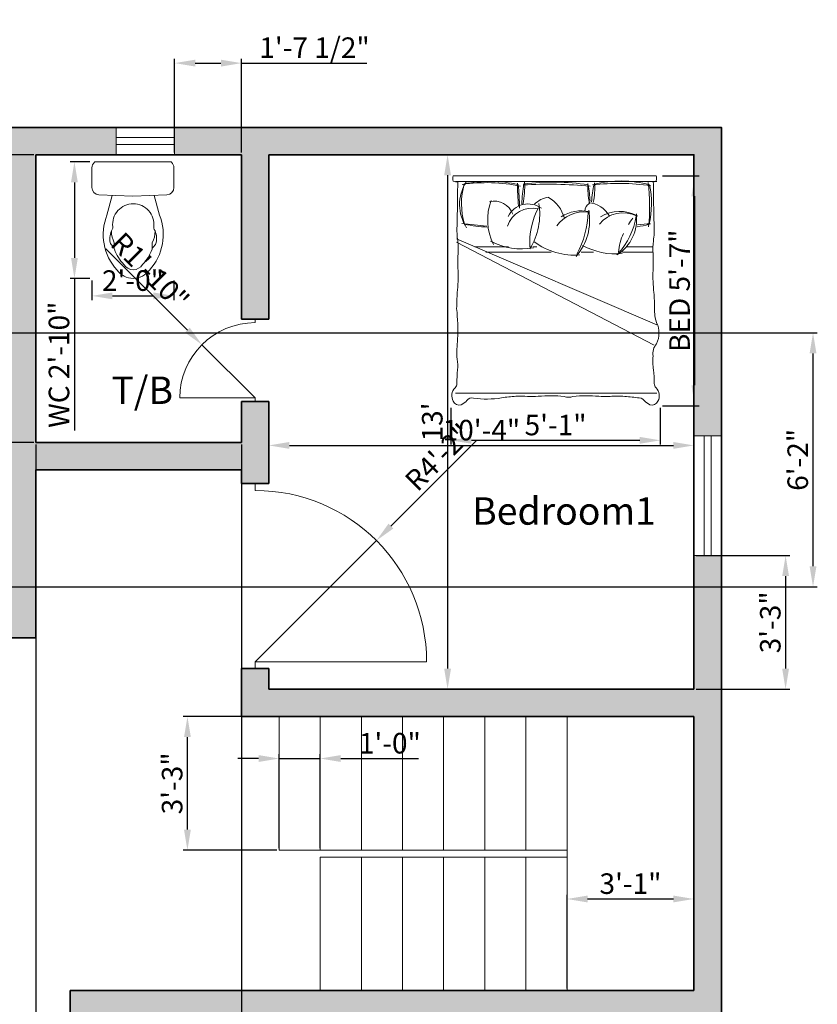
# Model space of a CAD drawing. Units: inches. Extents: x 2129 to 3258, y 1851 to 3021.
# Tile 7 of 10: x 2365 to 2598, y 2151 to 2439. Entities that reach past the tile are written whole.
import ezdxf

# ---------------------------------------------------------------- set-up
doc = ezdxf.new("R2010")
doc.units = ezdxf.units.IN
doc.linetypes.add('ACAD_ISO03W100', pattern=[30, 12, -18])
for name, color, linetype, lineweight in [('A-ANNO-DIMS', 2, 'Continuous', 18), ('A-AREA-IDEN', 7, 'Continuous', 20), ('A-DOOR', 4, 'Continuous', 18), ('A-FLOR-FIXT', 9, 'Continuous', 18), ('A-FLOR-STRS', 7, 'Continuous', 20), ('A-FURN', 8, 'Continuous', 18), ('A-GLAZ', 4, 'Continuous', 18), ('A-WALL', 7, 'Continuous', 35), ('A-WALL-OVHD', 8, 'ACAD_ISO03W100', 18)]:
    doc.layers.add(name, color=color, linetype=linetype, lineweight=lineweight)
doc.layers.add('A-WALL-PATT', color=32, linetype='Continuous', lineweight=13, true_color=0xcd6928)
doc.styles.get("Standard").update_dxf_attribs({"font": 'arial.ttf'})
doc.dimstyles.new('ISO-25', dxfattribs={"dimtxt": 6, "dimasz": 6, "dimexe": 1.25, "dimexo": 0.625, "dimtad": 1, "dimdec": 1, "dimlunit": 3, "dimtxsty": 'Standard', "dimcen": 2.5, "dimclrd": 5, "dimclre": 5, "dimadec": 0, "dimazin": 0, "dimtfac": 1, "dimtdec": 1, "dimtmove": 0, "dimatfit": 3, "dimfxl": 1, "dimarcsym": 0})

# ---------------------------------------------------------------- blocks, each defined once
blk = doc.blocks.new('A$C1308471B')
at = {"ltscale": 20}
for p, q in [((0, 0.4607), (0, 0.0186)), ((0.0354, 0.4793), (0.1495, 0.4793)), ((0.2013, 0.2397), (0.1923, 0.4384)), ((0.1957, 0.3639), (0.3109, 0.3953)), ((0.5021, 0.3528), (0.4724, 0.3528)), ((0.4982, 0.3575), (0.4822, 0.3709)), ((0.2013, 0.2397), (0.1923, 0.0409)), ((0.1959, 0.1193), (0.3109, 0.0879)), ((0.5021, 0.1304), (0.4724, 0.1304)), ((0.4982, 0.1257), (0.4822, 0.1123)), ((0.0354, 0), (0.1495, 0))]:
    blk.add_line(p, q, dxfattribs=at)
for centre, radius, start, end in [((0.006, 0.4607), 0.006, 136.52689, 180), ((0.0354, 0.4328), 0.0465, 90, 136.52689), ((0.1495, 0.4365), 0.0429, 2.57554, 90), ((0.4248, 0.1104), 0.3068, 47.41345, 111.79241), ((0.3654, 0.2416), 0.1206, 83.35226, 180), ((0.3823, 0.3868), 0.0255, 263.35226, 298.57415), ((0.4494, 0.2636), 0.1148, 79.39683, 118.57415), ((0.405, 0.2159), 0.153, 63.50202, 90.45216), ((0.4658, 0.3513), 0.0255, 50, 79.39683), ((0.5146, 0.377), 0.0255, 230, 251.38812), ((0.5021, 0.3273), 0.0255, 70.3751, 90), ((0.4248, 0.1104), 0.2558, 46.61198, 70.3751), ((0.5654, 0.2416), 0.065, 0, 57.29738), ((0.5654, 0.2416), 0.116, 0, 54.71147), ((0.3654, 0.2416), 0.1206, 180, 276.64774), ((0.5654, 0.2416), 0.065, 302.70262, 0), ((0.5654, 0.2416), 0.116, 305.28853, 0), ((0.4248, 0.3728), 0.2558, 289.6249, 313.38802), ((0.4248, 0.3728), 0.3068, 248.20759, 312.58655), ((0.3823, 0.0964), 0.0255, 61.42585, 96.64774), ((0.4494, 0.2196), 0.1148, 241.42585, 280.60317), ((0.405, 0.2673), 0.153, 269.54784, 296.49798), ((0.5146, 0.1062), 0.0255, 108.61188, 130), ((0.5021, 0.1559), 0.0255, 270, 289.6249), ((0.4658, 0.1319), 0.0255, 280.60317, 310), ((0.006, 0.0186), 0.006, 180, 223.47311), ((0.0354, 0.0465), 0.0465, 223.47311, 270), ((0.1495, 0.0429), 0.0429, 270, 357.42446)]:
    blk.add_arc(centre, radius, start, end, dxfattribs=at)
blk = doc.blocks.new('bed 1- king size')
at = {"color": 0}
for p, q in [((-0.9487, -0.0777), (0.9323, -0.0777)), ((-0.9394, -0.6151), (0.9323, -1.4177)), ((-0.9394, -0.6451), (0.9066, -1.6065)), ((-0.7682, -0.6873), (-0.4547, -0.6873)), ((-0.2254, -0.6873), (-0.1884, -0.6873)), ((0.6495, -0.6873), (0.8951, -0.6873)), ((-0.6659, -0.7381), (-0.0555, -0.7381)), ((0.2254, -0.7381), (0.3384, -0.7381)), ((0.6103, -0.7381), (0.8953, -0.7381)), ((-0.9487, -2.0547), (0.9323, -2.0547))]:
    blk.add_line(p, q, dxfattribs=at)
blk.add_lwpolyline([(0.898, -0.0829, 0.098699), (0.9236, -0.072, 0.222522), (0.9236, -0.0243), (-0.9705, -0.0243, 0.171621), (-0.9716, -0.0739, 0.102495), (-0.9268, -0.0829, 0.015571), (-0.9293, -0.2659, 0.00267), (-0.9341, -0.4944, 0.058958), (-0.9274, -0.6315, -0.038458), (-0.9248, -0.7552, 0.025508), (-0.9248, -0.9094, -0.039412), (-0.9326, -1.1154, 0.016498), (-0.9382, -1.2654, -0.035771), (-0.9288, -1.5502, 0.045388), (-0.9341, -1.7389, -0.080578), (-0.9295, -1.837, 0.026504), (-0.9362, -1.9656, -0.211134), (-0.9531, -2.0066, 0.329446), (-0.9701, -2.1314, 0.37589), (-0.8958, -2.1647, 0.123892), (-0.8425, -2.1233, -0.342539), (-0.78, -2.1029, 0.07104), (-0.5197, -2.1004, -0.036442), (-0.3847, -2.0853, -0.046791), (-0.2759, -2.0873, 0.023628), (-0.1759, -2.0852, -0.055897), (0.0662, -2.0877, 0.053528), (0.1067, -2.0945, 0.053528), (0.1472, -2.0877, -0.055897), (0.3893, -2.0852, 0.026973), (0.4769, -2.0873, -0.036947), (0.6147, -2.0853, -0.036442), (0.7497, -2.1004, -0.281256), (0.8137, -2.1233, -0.521995), (0.8137, -2.1233, 0.123892), (0.867, -2.1647, 0.37589), (0.9413, -2.1314, 0.329446), (0.9243, -2.0066, -0.211134), (0.9074, -1.9656, 0.026504), (0.9007, -1.837, -0.06219), (0.896, -1.7098, -0.218233), (0.9286, -1.5937, 0.123513), (0.9499, -1.4937, 0.129887), (0.9293, -1.3978, -0.095063), (0.9094, -1.2654, 0.016498), (0.9038, -1.1154, -0.039412), (0.896, -0.9094, 0.025508), (0.896, -0.7552, -0.038458), (0.8986, -0.6315, 0.058958), (0.9053, -0.4944, 0.00267), (0.9005, -0.2659, 0.015571)], format="xyb", close=True, dxfattribs=at)
for centre, radius, start, end in [((-0.5221, -0.2938), 0.3887, 147.50996, 213.83359), ((-0.6569, -1.6774), 1.5884, 78.54853, 98.3029), ((-0.6323, -1.3651), 1.2872, 78.01421, 100.51248), ((-1.2482, -0.1161), 0.9455, 349.58899, 2.04467), ((-0.04, -2.1818), 2.0978, 80.93396, 97.42659), ((0.5931, -1.1167), 1.0433, 75.01813, 103.73916), ((-1.0492, -0.3038), 1.9129, 354.09351, 6.47074), ((-0.2311, -0.2827), 0.6619, 163.92635, 197.14087), ((2.5431, -0.0869), 2.9129, 180.10628, 184.33117), ((-1.857, -0.3037), 1.5051, 359.15358, 7.55329), ((0.7071, -0.2897), 1.0355, 169.53013, 179.93405), ((-0.0818, -4.0689), 3.9654, 84.36579, 93.39687), ((1.0242, -0.1263), 0.7375, 177.82608, 191.47674), ((-0.6896, -0.2953), 0.9974, 1.8337, 10.6945), ((1.0572, -0.2894), 0.7358, 165.3434, 178.38757), ((0.5721, -2.1074), 2.0115, 81.37136, 96.91703), ((-0.3946, -0.1329), 0.7459, 349.16666, 3.12297), ((0.0089, -0.2863), 0.8722, 347.31751, 11.74345), ((-0.1358, -0.4371), 0.5128, 159.30257, 206.50263), ((-0.5846, -0.4421), 0.1803, 18.93869, 104.67251), ((-0.0546, -0.4435), 0.2189, 96.89924, 136.04208), ((-0.2438, -0.5051), 0.323, 15.40176, 59.7122), ((-0.2301, -0.5756), 0.2484, 78.04126, 160.83423), ((-0.2688, -0.4962), 0.2082, 54.16706, 153.84213), ((0.4039, -0.6426), 0.6595, 151.04555, 184.14969), ((-0.7873, -0.3825), 0.6248, 328.65419, 9.19769), ((0.2545, -0.6795), 0.3178, 83.56066, 144.28529), ((0.2294, -0.7137), 0.3612, 78.40806, 122.00775), ((-0.2123, -0.4404), 0.5157, 319.13389, 10.52989), ((-0.5982, -0.336), 0.8889, 331.60495, 358.1749), ((0.347, -0.3604), 0.0899, 120.11341, 175.89742), ((0.2786, -0.5137), 0.2374, 28.19956, 86.50605), ((0.5856, -0.7025), 0.345, 61.64039, 121.33448), ((0.6148, -0.6485), 0.2783, 61.88763, 141.87071), ((0.3458, -0.4294), 0.3969, 302.32623, 7.00001), ((0.0793, -0.3025), 0.6649, 317.32013, 351.4624), ((1.163, -0.8025), 0.5939, 139.95083, 146.95102), ((-1.8444, -10.4721), 10.046, 83.21322, 84.54762), ((-0.6059, 0.7469), 1.2515, 258.11692, 267.88493), ((0.6944, 0.0492), 0.5523, 275.44698, 287.41987), ((0.8799, -1.1936), 0.7214, 90.64318, 100.27066), ((-0.3293, -0.0779), 0.6301, 242.38587, 279.89508), ((0.1632, -0.137), 0.6293, 233.2201, 274.49725), ((1.163, -0.8025), 0.5939, 156.29818, 173.85386), ((0.5459, -0.118), 0.637, 240.94673, 275.46705)]:
    blk.add_arc(centre, radius, start, end, dxfattribs=at)
blk = doc.blocks.new('*D11')
at = {"layer": 'A-ANNO-DIMS', "color": 0, "lineweight": -2, "transparency": 16777216}
for p, q in [((2437.93, 2315.01), (2437.93, 2315.63)), ((2443.93, 2314.38), (2555.93, 2314.38)), ((2561.93, 2315.01), (2561.93, 2315.63))]:
    blk.add_line(p, q, dxfattribs=at)
at = {"layer": 'A-ANNO-DIMS', "color": 0, "transparency": 16777216}
for points in [[(2443.93, 2315.38), (2443.93, 2313.38), (2437.93, 2314.38)], [(2555.93, 2315.38), (2555.93, 2313.38), (2561.93, 2314.38)]]:
    blk.add_solid(points, dxfattribs=at)
at = {"layer": 'Defpoints', "color": 0, "transparency": 16777216}
for p in [(2437.93, 2314.38), (2561.93, 2314.38), (2561.93, 2314.38)]:
    blk.add_point(p, dxfattribs=at)
at = {"layer": 'A-ANNO-DIMS', "color": 0, "transparency": 16777216, "insert": (2499.93, 2318.07), "char_height": 6, "attachment_point": 5}
blk.add_mtext('10\'-4"', dxfattribs=at)
blk = doc.blocks.new('*D12')
at = {"layer": 'A-ANNO-DIMS', "color": 0, "lineweight": -2, "transparency": 16777216}
for p, q in [((2480.84, 2399.23), (2491.31, 2399.23)), ((2490.06, 2393.23), (2490.06, 2249.23)), ((2480.84, 2243.23), (2491.31, 2243.23))]:
    blk.add_line(p, q, dxfattribs=at)
at = {"layer": 'A-ANNO-DIMS', "color": 0, "transparency": 16777216}
for points in [[(2489.06, 2393.23), (2491.06, 2393.23), (2490.06, 2399.23)], [(2489.06, 2249.23), (2491.06, 2249.23), (2490.06, 2243.23)]]:
    blk.add_solid(points, dxfattribs=at)
at = {"layer": 'Defpoints', "color": 0, "transparency": 16777216}
for p in [(2480.22, 2399.23), (2480.22, 2243.23), (2490.06, 2243.23)]:
    blk.add_point(p, dxfattribs=at)
at = {"layer": 'A-ANNO-DIMS', "color": 0, "transparency": 16777216, "insert": (2486.37, 2321.23), "char_height": 6, "attachment_point": 5, "rotation": 90}
blk.add_mtext("13'", dxfattribs=at)
blk = doc.blocks.new('WIN-PLAN-35')
for p, q in [((0, 5), (35, 5)), ((0, 3), (35, 3))]:
    blk.add_line(p, q)
blk.add_lwpolyline([(0, 8), (35, 8), (35, 0), (0, 0)], close=True)
blk = doc.blocks.new('WIN-PLAN-17')
for p, q in [((0, 5), (17.03, 5)), ((0, 3), (17.03, 3))]:
    blk.add_line(p, q)
blk.add_lwpolyline([(0, 8), (17.03, 8), (17.03, 0), (0, 0)], close=True)
blk = doc.blocks.new('*D68')
at = {"layer": 'A-ANNO-DIMS', "color": 5, "lineweight": -2, "transparency": 16777216}
for p, q in [((2552.75, 2393.11), (2563.45, 2393.11)), ((2562.2, 2331.95), (2562.2, 2387.11)), ((2552.75, 2325.95), (2563.45, 2325.95))]:
    blk.add_line(p, q, dxfattribs=at)
at = {"layer": 'A-ANNO-DIMS', "color": 5, "transparency": 16777216}
for points in [[(2561.2, 2387.11), (2563.2, 2387.11), (2562.2, 2393.11)], [(2561.2, 2331.95), (2563.2, 2331.95), (2562.2, 2325.95)]]:
    blk.add_solid(points, dxfattribs=at)
at = {"layer": 'Defpoints', "color": 0, "transparency": 16777216}
for p in [(2552.13, 2393.11), (2562.2, 2393.11), (2552.13, 2325.95)]:
    blk.add_point(p, dxfattribs=at)
at = {"layer": 'A-ANNO-DIMS', "color": 0, "transparency": 16777216, "insert": (2558.52, 2359.53), "char_height": 6, "attachment_point": 5, "rotation": 90}
blk.add_mtext('BED 5\'-7"', dxfattribs=at)
blk = doc.blocks.new('*D69')
at = {"layer": 'A-ANNO-DIMS', "color": 5, "lineweight": -2, "transparency": 16777216}
for p, q in [((2491.01, 2325.32), (2491.01, 2314.62)), ((2552.13, 2325.32), (2552.13, 2314.62)), ((2497.01, 2315.87), (2546.13, 2315.87))]:
    blk.add_line(p, q, dxfattribs=at)
at = {"layer": 'A-ANNO-DIMS', "color": 5, "transparency": 16777216}
for points in [[(2497.01, 2316.87), (2497.01, 2314.87), (2491.01, 2315.87)], [(2546.13, 2316.87), (2546.13, 2314.87), (2552.13, 2315.87)]]:
    blk.add_solid(points, dxfattribs=at)
at = {"layer": 'Defpoints', "color": 0, "transparency": 16777216}
for p in [(2491.01, 2325.95), (2552.13, 2325.95), (2552.13, 2315.87)]:
    blk.add_point(p, dxfattribs=at)
at = {"layer": 'A-ANNO-DIMS', "color": 0, "transparency": 16777216, "insert": (2521.57, 2319.56), "char_height": 6, "attachment_point": 5}
blk.add_mtext('5\'-1"', dxfattribs=at)
blk = doc.blocks.new('*D74')
at = {"layer": 'A-ANNO-DIMS', "color": 5, "lineweight": -2, "transparency": 16777216}
for p, q in [((2385.67, 2397.15), (2379.94, 2397.15)), ((2381.19, 2391.15), (2381.19, 2369.14)), ((2385.67, 2363.14), (2379.94, 2363.14)), ((2381.19, 2363.14), (2381.19, 2318.74))]:
    blk.add_line(p, q, dxfattribs=at)
at = {"layer": 'A-ANNO-DIMS', "color": 5, "transparency": 16777216}
for points in [[(2380.19, 2391.15), (2382.19, 2391.15), (2381.19, 2397.15)], [(2380.19, 2369.14), (2382.19, 2369.14), (2381.19, 2363.14)]]:
    blk.add_solid(points, dxfattribs=at)
at = {"layer": 'Defpoints', "color": 0, "transparency": 16777216}
for p in [(2386.29, 2397.15), (2381.19, 2363.14), (2386.29, 2363.14)]:
    blk.add_point(p, dxfattribs=at)
at = {"layer": 'A-ANNO-DIMS', "color": 0, "transparency": 16777216, "insert": (2377.46, 2337.94), "char_height": 6, "attachment_point": 5, "rotation": 90}
blk.add_mtext('WC 2\'-10"', dxfattribs=at)
blk = doc.blocks.new('*D75')
at = {"layer": 'A-ANNO-DIMS', "color": 5, "lineweight": -2, "transparency": 16777216}
for p, q in [((2386.29, 2362.51), (2386.29, 2356.78)), ((2410.22, 2362.51), (2410.22, 2356.78)), ((2392.29, 2358.03), (2404.22, 2358.03))]:
    blk.add_line(p, q, dxfattribs=at)
at = {"layer": 'A-ANNO-DIMS', "color": 5, "transparency": 16777216}
for points in [[(2392.29, 2359.03), (2392.29, 2357.03), (2386.29, 2358.03)], [(2404.22, 2359.03), (2404.22, 2357.03), (2410.22, 2358.03)]]:
    blk.add_solid(points, dxfattribs=at)
at = {"layer": 'Defpoints', "color": 0, "transparency": 16777216}
for p in [(2386.29, 2363.14), (2410.22, 2363.14), (2410.22, 2358.03)]:
    blk.add_point(p, dxfattribs=at)
at = {"layer": 'A-ANNO-DIMS', "color": 0, "transparency": 16777216, "insert": (2398.26, 2361.72), "char_height": 6, "attachment_point": 5}
blk.add_mtext('2\'-0"', dxfattribs=at)
blk = doc.blocks.new('*D91')
at = {"layer": 'A-ANNO-DIMS', "color": 5, "lineweight": -2, "transparency": 16777216}
for p, q in [((2369.93, 2314.61), (2369.93, 1851.23)), ((2429.93, 2314.61), (2429.93, 1851.23)), ((2375.93, 1852.48), (2423.93, 1852.48))]:
    blk.add_line(p, q, dxfattribs=at)
at = {"layer": 'A-ANNO-DIMS', "color": 5, "transparency": 16777216}
for points in [[(2375.93, 1853.48), (2375.93, 1851.48), (2369.93, 1852.48)], [(2423.93, 1853.48), (2423.93, 1851.48), (2429.93, 1852.48)]]:
    blk.add_solid(points, dxfattribs=at)
at = {"layer": 'Defpoints', "color": 0, "transparency": 16777216}
for p in [(2369.93, 2315.23), (2429.93, 2315.23), (2429.93, 1852.48)]:
    blk.add_point(p, dxfattribs=at)
at = {"layer": 'A-ANNO-DIMS', "color": 0, "transparency": 16777216, "insert": (2399.93, 1856.17), "char_height": 6, "attachment_point": 5}
blk.add_mtext('5\'-0"', dxfattribs=at)
blk = doc.blocks.new('*D92')
at = {"layer": 'A-ANNO-DIMS', "color": 5, "lineweight": -2, "transparency": 16777216}
for p, q in [((2369.3, 2399.23), (2157.93, 2399.23)), ((2159.18, 2321.23), (2159.18, 2393.23)), ((2369.3, 2315.23), (2157.93, 2315.23))]:
    blk.add_line(p, q, dxfattribs=at)
at = {"layer": 'A-ANNO-DIMS', "color": 5, "transparency": 16777216}
for points in [[(2158.18, 2393.23), (2160.18, 2393.23), (2159.18, 2399.23)], [(2158.18, 2321.23), (2160.18, 2321.23), (2159.18, 2315.23)]]:
    blk.add_solid(points, dxfattribs=at)
at = {"layer": 'Defpoints', "color": 0, "transparency": 16777216}
for p in [(2159.18, 2399.23), (2369.93, 2399.23), (2369.93, 2315.23)]:
    blk.add_point(p, dxfattribs=at)
at = {"layer": 'A-ANNO-DIMS', "color": 0, "transparency": 16777216, "insert": (2155.49, 2357.23), "char_height": 6, "attachment_point": 5, "rotation": 90}
blk.add_mtext('7\'-0"', dxfattribs=at)
blk = doc.blocks.new('*D94')
at = {"layer": 'A-ANNO-DIMS', "color": 5, "lineweight": -2, "transparency": 16777216}
for p, q in [((2440.28, 2235.23), (2412.91, 2235.23)), ((2414.16, 2202.23), (2414.16, 2229.23)), ((2440.28, 2196.23), (2412.91, 2196.23))]:
    blk.add_line(p, q, dxfattribs=at)
at = {"layer": 'A-ANNO-DIMS', "color": 5, "transparency": 16777216}
for points in [[(2413.16, 2229.23), (2415.16, 2229.23), (2414.16, 2235.23)], [(2413.16, 2202.23), (2415.16, 2202.23), (2414.16, 2196.23)]]:
    blk.add_solid(points, dxfattribs=at)
at = {"layer": 'Defpoints', "color": 0, "transparency": 16777216}
for p in [(2414.16, 2235.23), (2440.91, 2235.23), (2440.91, 2196.23)]:
    blk.add_point(p, dxfattribs=at)
at = {"layer": 'A-ANNO-DIMS', "color": 0, "transparency": 16777216, "insert": (2410.47, 2215.73), "char_height": 6, "attachment_point": 5, "rotation": 90}
blk.add_mtext('3\'-3"', dxfattribs=at)
blk = doc.blocks.new('*D95')
at = {"layer": 'A-ANNO-DIMS', "color": 5, "lineweight": -2, "transparency": 16777216}
for p, q in [((2434.91, 2222.98), (2428.91, 2222.98)), ((2440.91, 2196.86), (2440.91, 2224.23)), ((2440.91, 2222.98), (2452.91, 2222.98)), ((2452.91, 2196.86), (2452.91, 2224.23)), ((2458.91, 2222.98), (2481.54, 2222.98))]:
    blk.add_line(p, q, dxfattribs=at)
at = {"layer": 'A-ANNO-DIMS', "color": 5, "transparency": 16777216}
for points in [[(2434.91, 2223.98), (2434.91, 2221.98), (2440.91, 2222.98)], [(2458.91, 2223.98), (2458.91, 2221.98), (2452.91, 2222.98)]]:
    blk.add_solid(points, dxfattribs=at)
at = {"layer": 'Defpoints', "color": 0, "transparency": 16777216}
for p in [(2452.91, 2222.98), (2440.91, 2196.23), (2452.91, 2196.23)]:
    blk.add_point(p, dxfattribs=at)
at = {"layer": 'A-ANNO-DIMS', "color": 0, "transparency": 16777216, "insert": (2473.22, 2226.67), "char_height": 6, "attachment_point": 5}
blk.add_mtext('1\'-0"', dxfattribs=at)
blk = doc.blocks.new('*D96')
at = {"layer": 'A-ANNO-DIMS', "color": 5, "lineweight": -2, "transparency": 16777216}
for p, q in [((2524.91, 2155.86), (2524.91, 2183.23)), ((2530.91, 2181.98), (2555.93, 2181.98)), ((2561.93, 2155.86), (2561.93, 2183.23))]:
    blk.add_line(p, q, dxfattribs=at)
at = {"layer": 'A-ANNO-DIMS', "color": 5, "transparency": 16777216}
for points in [[(2530.91, 2182.98), (2530.91, 2180.98), (2524.91, 2181.98)], [(2555.93, 2182.98), (2555.93, 2180.98), (2561.93, 2181.98)]]:
    blk.add_solid(points, dxfattribs=at)
at = {"layer": 'Defpoints', "color": 0, "transparency": 16777216}
for p in [(2561.93, 2181.98), (2524.91, 2155.23), (2561.93, 2155.23)]:
    blk.add_point(p, dxfattribs=at)
at = {"layer": 'A-ANNO-DIMS', "color": 0, "transparency": 16777216, "insert": (2543.42, 2185.68), "char_height": 6, "attachment_point": 5}
blk.add_mtext('3\'-1"', dxfattribs=at)
blk = doc.blocks.new('*D98')
at = {"layer": 'A-ANNO-DIMS', "color": 5, "lineweight": -2, "transparency": 16777216}
for p, q in [((2230.55, 2347.23), (2597.93, 2347.23)), ((2596.68, 2279.1), (2596.68, 2341.23)), ((2230.55, 2273.1), (2597.93, 2273.1))]:
    blk.add_line(p, q, dxfattribs=at)
at = {"layer": 'A-ANNO-DIMS', "color": 5, "transparency": 16777216}
for points in [[(2595.68, 2341.23), (2597.68, 2341.23), (2596.68, 2347.23)], [(2595.68, 2279.1), (2597.68, 2279.1), (2596.68, 2273.1)]]:
    blk.add_solid(points, dxfattribs=at)
at = {"layer": 'Defpoints', "color": 0, "transparency": 16777216}
for p in [(2229.93, 2347.23), (2596.68, 2347.23), (2229.93, 2273.1)]:
    blk.add_point(p, dxfattribs=at)
at = {"layer": 'A-ANNO-DIMS', "color": 0, "transparency": 16777216, "insert": (2592.99, 2310.17), "char_height": 6, "attachment_point": 5, "rotation": 90}
blk.add_mtext('6\'-2"', dxfattribs=at)
blk = doc.blocks.new('*D107')
at = {"layer": 'A-ANNO-DIMS', "color": 5, "lineweight": -2, "transparency": 16777216}
for p, q in [((2410.42, 2399.86), (2410.42, 2427.23)), ((2416.42, 2425.98), (2423.93, 2425.98)), ((2429.93, 2399.86), (2429.93, 2427.23)), ((2429.93, 2425.98), (2466.54, 2425.98))]:
    blk.add_line(p, q, dxfattribs=at)
at = {"layer": 'A-ANNO-DIMS', "color": 5, "transparency": 16777216}
for points in [[(2416.42, 2426.98), (2416.42, 2424.98), (2410.42, 2425.98)], [(2423.93, 2426.98), (2423.93, 2424.98), (2429.93, 2425.98)]]:
    blk.add_solid(points, dxfattribs=at)
at = {"layer": 'Defpoints', "color": 0, "transparency": 16777216}
for p in [(2429.93, 2425.98), (2410.42, 2399.23), (2429.93, 2399.23)]:
    blk.add_point(p, dxfattribs=at)
at = {"layer": 'A-ANNO-DIMS', "color": 0, "transparency": 16777216, "insert": (2451.24, 2429.71), "char_height": 6, "attachment_point": 5}
blk.add_mtext('1\'-7 1/2"', dxfattribs=at)
blk = doc.blocks.new('*D113')
at = {"layer": 'A-ANNO-DIMS', "color": 5, "lineweight": -2, "transparency": 16777216}
for p, q in [((2562.55, 2282.22), (2589.93, 2282.22)), ((2588.68, 2276.22), (2588.68, 2249.23)), ((2562.55, 2243.23), (2589.93, 2243.23))]:
    blk.add_line(p, q, dxfattribs=at)
at = {"layer": 'A-ANNO-DIMS', "color": 5, "transparency": 16777216}
for points in [[(2587.68, 2276.22), (2589.68, 2276.22), (2588.68, 2282.22)], [(2587.68, 2249.23), (2589.68, 2249.23), (2588.68, 2243.23)]]:
    blk.add_solid(points, dxfattribs=at)
at = {"layer": 'Defpoints', "color": 0, "transparency": 16777216}
for p in [(2561.93, 2282.22), (2561.93, 2243.23), (2588.68, 2243.23)]:
    blk.add_point(p, dxfattribs=at)
at = {"layer": 'A-ANNO-DIMS', "color": 0, "transparency": 16777216, "insert": (2584.99, 2262.73), "char_height": 6, "attachment_point": 5, "rotation": 90}
blk.add_mtext('3\'-3"', dxfattribs=at)
blk = doc.blocks.new('*D135')
at = {"layer": 'A-ANNO-DIMS', "color": 5, "lineweight": -2, "transparency": 16777216}
for p, q in [((2498.61, 2315.91), (2473.53, 2290.83)), ((2433.93, 2251.23), (2469.28, 2286.59))]:
    blk.add_line(p, q, dxfattribs=at)
at = {"layer": 'A-ANNO-DIMS', "color": 5, "transparency": 16777216}
blk.add_solid([(2472.82, 2291.54), (2474.23, 2290.13), (2469.28, 2286.59)], dxfattribs=at)
at = {"layer": 'Defpoints', "color": 0, "transparency": 16777216}
for p in [(2469.28, 2286.59), (2433.93, 2251.23)]:
    blk.add_point(p, dxfattribs=at)
at = {"layer": 'A-ANNO-DIMS', "color": 0, "transparency": 16777216, "insert": (2487.92, 2310.38), "char_height": 6, "attachment_point": 5, "rotation": 45.0003}
blk.add_mtext('R4\'-2"', dxfattribs=at)
blk = doc.blocks.new('*D139')
at = {"layer": 'A-ANNO-DIMS', "color": 5, "lineweight": -2, "transparency": 16777216}
for p, q in [((2390.38, 2371.81), (2414.13, 2348.04)), ((2433.93, 2328.23), (2418.38, 2343.79))]:
    blk.add_line(p, q, dxfattribs=at)
at = {"layer": 'A-ANNO-DIMS', "color": 5, "transparency": 16777216}
blk.add_solid([(2414.84, 2348.75), (2413.43, 2347.33), (2418.38, 2343.79)], dxfattribs=at)
at = {"layer": 'Defpoints', "color": 0, "transparency": 16777216}
for p in [(2418.38, 2343.79), (2433.93, 2328.23)]:
    blk.add_point(p, dxfattribs=at)
at = {"layer": 'A-ANNO-DIMS', "color": 0, "transparency": 16777216, "insert": (2402.74, 2364.65), "char_height": 6, "attachment_point": 5, "rotation": 314.9864}
blk.add_mtext('R1\'-10"', dxfattribs=at)

msp = doc.modelspace()

# ---------------------------------------------------------------- hatches: boundary and pattern name
at = {"layer": 'A-WALL-PATT'}
h = msp.add_hatch(color=256, dxfattribs=at)
h.dxf.hatch_style = 1
h.paths.add_polyline_path([(2393.39, 2407.23), (2185.93, 2407.23), (2185.93, 2394.06), (2193.93, 2394.06), (2193.93, 2399.23), (2361.93, 2399.23), (2361.93, 2355.23), (2361.93, 2347.23), (2361.93, 2258.25), (2369.93, 2258.25), (2369.93, 2307.23), (2429.93, 2307.23), (2429.93, 2303.23), (2437.93, 2303.23), (2437.93, 2327.23), (2429.93, 2327.23), (2429.93, 2315.23), (2369.93, 2315.23), (2369.93, 2399.23), (2393.39, 2399.23)])
h.paths.add_polyline_path([(2569.93, 2407.23), (2410.42, 2407.23), (2410.42, 2399.23), (2429.93, 2399.23), (2429.93, 2351.23), (2437.93, 2351.23), (2437.93, 2399.23), (2561.93, 2399.23), (2561.93, 2317.22), (2569.93, 2317.22)])
h.paths.add_polyline_path([(2569.93, 2282.22), (2561.93, 2282.22), (2561.93, 2243.23), (2437.93, 2243.23), (2437.93, 2249.23), (2429.93, 2249.23), (2429.93, 2235.23), (2561.93, 2235.23), (2561.93, 2155.23), (2379.93, 2155.23), (2379.93, 2147.23), (2385.93, 2147.23), (2385.93, 2141.23), (2393.93, 2141.23), (2393.93, 2147.23), (2469.93, 2147.23), (2469.93, 2111.23), (2477.93, 2111.23), (2477.93, 2147.23), (2561.93, 2147.23), (2561.93, 2129.53), (2569.93, 2129.53)])
h.paths.add_polyline_path([(2569.93, 2112.5), (2561.93, 2112.5), (2561.93, 2063.23), (2477.93, 2063.23), (2477.93, 2069.23), (2469.93, 2069.23), (2469.93, 2063.23), (2445.93, 2063.23), (2445.93, 2055.23), (2561.93, 2055.23), (2561.93, 1951.04), (2569.93, 1951.04)])
h.paths.add_polyline_path([(2569.93, 1916.04), (2561.93, 1916.04), (2561.93, 1887.23), (2393.93, 1887.23), (2393.93, 2055.23), (2399.93, 2055.23), (2399.93, 2063.23), (2393.93, 2063.23), (2393.93, 2087.23), (2385.93, 2087.23), (2385.93, 1887.23), (2385.93, 1879.23), (2569.93, 1879.23)])
h.paths.add_polyline_path([(2193.93, 2147.23), (2289.93, 2147.23), (2289.93, 2155.23), (2193.93, 2155.23), (2193.93, 2170.77), (2185.93, 2170.77), (2185.93, 2056.85), (2193.93, 2056.85)])
h.paths.add_polyline_path([(2193.93, 2021.85), (2185.93, 2021.85), (2185.93, 1959.23), (2222.56, 1959.23), (2222.56, 1967.23), (2193.93, 1967.23)])
h.paths.add_polyline_path([(2307.93, 1967.23), (2257.56, 1967.23), (2257.56, 1959.23), (2307.93, 1959.23)])
h.paths.add_polyline_path([(2255.61, 2368.18), (2321.09, 2368.18), (2321.09, 2384.66), (2255.61, 2384.66)], flags=25)
h.paths.add_polyline_path([(2282.89, 2032.34), (2325.27, 2032.34), (2325.27, 2051.27), (2282.89, 2051.27)], flags=9)
h.paths.add_polyline_path([(2404.09, 1945.18), (2463.36, 1945.18), (2463.36, 1961.66), (2404.09, 1961.66)], flags=25)
h.paths.add_polyline_path([(2494.41, 2286.84), (2553.68, 2286.84), (2553.68, 2303.32), (2494.41, 2303.32)], flags=9)
h.paths.add_polyline_path([(2389.71, 2321.98), (2411.09, 2321.98), (2411.09, 2338.47), (2389.71, 2338.47)], flags=25)
h.paths.add_polyline_path([(2219.41, 2162.82), (2258.18, 2162.82), (2258.18, 2179.3), (2219.41, 2179.3)], flags=9)
h.paths.add_polyline_path([(2249.68, 2306.23), (2298.12, 2306.23), (2298.12, 2323.98), (2249.68, 2323.98)], flags=25)
h = msp.add_hatch(color=256, dxfattribs=at)
h.dxf.hatch_style = 1
h.paths.add_polyline_path([(2193.93, 2288.35), (2185.93, 2288.35), (2185.93, 2205.77), (2193.93, 2205.77)])
h.paths.add_polyline_path([(2193.93, 2347.23), (2310.77, 2347.23), (2310.77, 2355.23), (2193.93, 2355.23), (2193.93, 2359.06), (2185.93, 2359.06), (2185.93, 2323.35), (2193.93, 2323.35)])
h.paths.add_polyline_path([(2314.44, 2244.01), (2314.44, 2257.94), (2302.07, 2257.94), (2302.07, 2244.01)], flags=9)
h.paths.add_polyline_path([(2255.61, 2368.18), (2321.09, 2368.18), (2321.09, 2384.66), (2255.61, 2384.66)], flags=9)
h.paths.add_polyline_path([(2282.89, 2032.34), (2325.27, 2032.34), (2325.27, 2051.27), (2282.89, 2051.27)], flags=9)
h.paths.add_polyline_path([(2404.09, 1945.18), (2463.36, 1945.18), (2463.36, 1961.66), (2404.09, 1961.66)], flags=9)
h.paths.add_polyline_path([(2494.41, 2286.84), (2553.68, 2286.84), (2553.68, 2303.32), (2494.41, 2303.32)], flags=9)
h.paths.add_polyline_path([(2389.71, 2321.98), (2411.09, 2321.98), (2411.09, 2338.47), (2389.71, 2338.47)], flags=9)
h.paths.add_polyline_path([(2219.41, 2162.82), (2258.18, 2162.82), (2258.18, 2179.3), (2219.41, 2179.3)], flags=9)
h.paths.add_polyline_path([(2249.68, 2306.23), (2298.12, 2306.23), (2298.12, 2323.98), (2249.68, 2323.98)], flags=9)

# ---------------------------------------------------------------- linework, layer by layer
at = {"layer": 'A-DOOR'}
for p, q in [((2433.93, 2351.23), (2433.93, 2350.23)), ((2433.93, 2328.23), (2411.93, 2328.23)), ((2433.93, 2327.23), (2433.93, 2328.23)), ((2433.93, 2303.23), (2433.93, 2301.23)), ((2433.93, 2249.23), (2433.93, 2251.23)), ((2433.93, 2251.23), (2483.93, 2251.23))]:
    msp.add_line(p, q, dxfattribs=at)
for centre, radius, start, end in [((2433.93, 2328.23), 22, 90, 180), ((2433.93, 2251.23), 50, 0, 90)]:
    msp.add_arc(centre, radius, start, end, dxfattribs=at)
at = {"layer": 'A-FLOR-STRS'}
for p, q in [((2440.91, 2235.23), (2440.91, 2196.23)), ((2452.91, 2235.23), (2452.91, 2196.23)), ((2464.91, 2235.23), (2464.91, 2196.23)), ((2476.91, 2235.23), (2476.91, 2196.23)), ((2488.91, 2196.23), (2488.91, 2235.23)), ((2500.91, 2235.23), (2500.91, 2196.23)), ((2512.91, 2235.23), (2512.91, 2196.23)), ((2524.91, 2235.23), (2524.91, 2194.23)), ((2524.91, 2196.23), (2440.91, 2196.23)), ((2524.91, 2194.23), (2452.91, 2194.23)), ((2452.91, 2194.23), (2452.91, 2155.23)), ((2464.91, 2194.23), (2464.91, 2155.23)), ((2476.91, 2194.23), (2476.91, 2155.23)), ((2488.91, 2194.23), (2488.91, 2155.23)), ((2500.91, 2194.23), (2500.91, 2155.23)), ((2512.91, 2194.23), (2512.91, 2155.23)), ((2524.91, 2194.23), (2524.91, 2155.23))]:
    msp.add_line(p, q, dxfattribs=at)
at = {"layer": 'A-WALL'}
for p, q in [((2369.93, 2399.23), (2369.93, 2315.23)), ((2429.93, 2399.23), (2429.93, 2351.23)), ((2437.93, 2399.23), (2437.93, 2351.23)), ((2437.93, 2399.23), (2561.93, 2399.23)), ((2429.93, 2351.23), (2437.93, 2351.23)), ((2429.93, 2327.23), (2437.93, 2327.23)), ((2429.93, 2327.23), (2429.93, 2315.23)), ((2437.93, 2327.23), (2437.93, 2303.23)), ((2369.93, 2315.23), (2429.93, 2315.23)), ((2369.93, 2307.23), (2429.93, 2307.23)), ((2369.93, 2307.23), (2369.93, 2258.25)), ((2429.93, 2307.23), (2429.93, 2303.23)), ((2429.93, 2303.23), (2437.93, 2303.23)), ((2361.93, 2258.25), (2369.93, 2258.25)), ((2437.93, 2249.23), (2429.93, 2249.23)), ((2429.93, 2249.23), (2429.93, 2235.23)), ((2437.93, 2249.23), (2437.93, 2243.23)), ((2437.93, 2243.23), (2561.93, 2243.23)), ((2429.93, 2235.23), (2561.93, 2235.23)), ((2561.93, 2235.23), (2561.93, 2155.23)), ((2379.93, 2147.23), (2379.93, 2155.23)), ((2379.93, 2155.23), (2561.93, 2155.23))]:
    msp.add_line(p, q, dxfattribs=at)
msp.add_lwpolyline([(2185.93, 2407.23), (2569.93, 2407.23), (2569.93, 1879.23), (2185.93, 1879.23)], close=True, dxfattribs=at)
for points in [[(2369.93, 2399.23), (2429.93, 2399.23)], [(2437.93, 2399.23), (2561.93, 2399.23), (2561.93, 2243.23)], [(2561.93, 2235.23), (2561.93, 2155.23)]]:
    msp.add_lwpolyline(points, dxfattribs=at)
at = {"layer": 'A-WALL-OVHD'}
msp.add_line((2289.93, 2155.23), (2379.93, 2155.23), dxfattribs=at)

# ---------------------------------------------------------------- block references
at = {"layer": 'A-FLOR-FIXT', "xscale": 49.91928435982494, "yscale": 49.91928435982494, "zscale": 49.91928435982494, "rotation": 269.9999999999996}
msp.add_blockref('A$C1308471B', (2386.29, 2397.15), dxfattribs=at)
at = {"layer": 'A-FURN', "xscale": 31.24411875038765, "yscale": 31.24411875038765, "zscale": 31.24411875038765}
msp.add_blockref('bed 1- king size', (2522.02, 2393.87), dxfattribs=at)
at = {"layer": 'A-GLAZ'}
msp.add_blockref('WIN-PLAN-17', (2393.39, 2399.24), dxfattribs=at)
at = {"layer": 'A-GLAZ', "rotation": 89.99999999999972}
msp.add_blockref('WIN-PLAN-35', (2569.93, 2282.22), dxfattribs=at)

# ---------------------------------------------------------------- texts
at = {"layer": 'A-AREA-IDEN', "char_height": 8, "attachment_point": 1}
for s, width, insert in [('T/B', 7.067, (2391.97, 2334.49)), ('{\\fArial|b1|i0|c0|p34;Bedroom1}', 58.4293, (2497.23, 2299.24))]:
    msp.add_mtext_dynamic_manual_height_columns(s, width=width, gutter_width=12.5, heights=[0], dxfattribs=dict(at, insert=insert))

# ---------------------------------------------------------------- dimensions: what is measured, and where the dimension line sits
at = {"layer": 'A-ANNO-DIMS'}
for base, p1, p2, override, picture, middle in [((2429.93, 2425.98), (2410.42, 2399.23), (2429.93, 2399.23), {"dimdec": 1, "dimlfac": 1, "dimrnd": 0, "dimzin": 1, "dimdsep": 46, "dimlunit": 4, "dimfrac": 2}, '*D107', (2451.24, 2429.71)), ((2410.22, 2358.03), (2386.29, 2363.14), (2410.22, 2363.14), {"dimdec": 1, "dimlfac": 1, "dimrnd": 0, "dimzin": 1, "dimdsep": 46, "dimlunit": 4, "dimfrac": 2}, '*D75', (2398.26, 2361.72)), ((2552.13, 2315.87), (2491.01, 2325.95), (2552.13, 2325.95), {"dimdec": 1, "dimlfac": 1, "dimrnd": 0, "dimzin": 1, "dimdsep": 46, "dimlunit": 4, "dimfrac": 2}, '*D69', (2521.57, 2319.56)), ((2561.93, 2314.38), (2437.93, 2314.38), (2561.93, 2314.38), {"dimclrd": 0, "dimclre": 0, "dimclrt": 0}, '*D11', (2499.93, 2318.07)), ((2429.93, 1852.48), (2369.93, 2315.23), (2429.93, 2315.23), {"dimdec": 1, "dimlfac": 1, "dimrnd": 0, "dimzin": 1, "dimdsep": 46, "dimlunit": 4, "dimfrac": 2}, '*D91', (2399.93, 1856.17)), ((2452.91, 2222.98), (2440.91, 2196.23), (2452.91, 2196.23), {"dimdec": 1, "dimlfac": 1, "dimrnd": 0, "dimzin": 1, "dimdsep": 46, "dimlunit": 4, "dimfrac": 2}, '*D95', (2473.22, 2226.67)), ((2561.93, 2181.98), (2524.91, 2155.23), (2561.93, 2155.23), {"dimdec": 1, "dimlfac": 1, "dimrnd": 0, "dimzin": 1, "dimdsep": 46, "dimlunit": 4, "dimfrac": 2}, '*D96', (2543.42, 2185.68))]:
    dim = msp.add_linear_dim(base=base, p1=p1, p2=p2, dimstyle='ISO-25', override=override, dxfattribs=at)
    dim.commit()
    dim.dimension.update_dxf_attribs({"geometry": picture, "text_midpoint": middle})
for base, p1, p2, angle, override, picture, middle in [((2159.18, 2399.23), (2369.93, 2315.23), (2369.93, 2399.23), 90, {"dimdec": 1, "dimlfac": 1, "dimrnd": 0, "dimzin": 1, "dimdsep": 46, "dimlunit": 4, "dimfrac": 2}, '*D92', (2155.49, 2357.23)), ((2490.06, 2243.23), (2480.22, 2399.23), (2480.22, 2243.23), 90, {"dimclrd": 0, "dimclre": 0, "dimclrt": 0}, '*D12', (2486.37, 2321.23)), ((2596.68, 2347.23), (2229.93, 2273.1), (2229.93, 2347.23), 90, {"dimdec": 1, "dimlfac": 1, "dimrnd": 0, "dimzin": 1, "dimdsep": 46, "dimlunit": 4, "dimfrac": 2}, '*D98', (2592.99, 2310.17)), ((2588.68, 2243.23), (2561.93, 2282.22), (2561.93, 2243.23), 270, {"dimdec": 1, "dimlfac": 1, "dimrnd": 0, "dimzin": 1, "dimdsep": 46, "dimlunit": 4, "dimfrac": 2}, '*D113', (2584.99, 2262.73)), ((2414.16, 2235.23), (2440.91, 2196.23), (2440.91, 2235.23), 90, {"dimdec": 1, "dimlfac": 1, "dimrnd": 0, "dimzin": 1, "dimdsep": 46, "dimlunit": 4, "dimfrac": 2}, '*D94', (2410.47, 2215.73))]:
    dim = msp.add_linear_dim(base=base, p1=p1, p2=p2, angle=angle, dimstyle='ISO-25', override=override, dxfattribs=at)
    dim.commit()
    dim.dimension.update_dxf_attribs({"geometry": picture, "text_midpoint": middle})
for base, p1, p2, angle, text, picture, middle in [((2381.19, 2363.14), (2386.29, 2397.15), (2386.29, 2363.14), 270, 'WC <>', '*D74', (2377.46, 2337.94)), ((2562.2, 2393.11), (2552.13, 2325.95), (2552.13, 2393.11), 90, 'BED <>', '*D68', (2558.52, 2359.53))]:
    dim = msp.add_linear_dim(base=base, p1=p1, p2=p2, angle=angle, text=text, dimstyle='ISO-25', override={"dimdec": 1, "dimlfac": 1, "dimrnd": 0, "dimzin": 1, "dimdsep": 46, "dimlunit": 4, "dimfrac": 2}, dxfattribs=at)
    dim.commit()
    dim.dimension.update_dxf_attribs({"geometry": picture, "text_midpoint": middle})
dim = msp.add_radius_dim(center=(2433.93, 2328.23), mpoint=(2418.38, 2343.79), dimstyle='ISO-25', override={"dimdec": 1, "dimlfac": 1, "dimrnd": 0, "dimzin": 1, "dimdsep": 46, "dimlunit": 4, "dimfrac": 2}, dxfattribs=at)
dim.commit()
dim.dimension.update_dxf_attribs({"geometry": '*D139', "text_midpoint": (2402.74, 2364.65)})
dim = msp.add_radius_dim(center=(2433.93, 2251.23), mpoint=(2469.28, 2286.59), dimstyle='ISO-25', override={"dimdec": 1, "dimlfac": 1, "dimrnd": 0, "dimzin": 1, "dimdsep": 46, "dimlunit": 4, "dimfrac": 2}, dxfattribs=at)
dim.commit()
dim.dimension.update_dxf_attribs({"geometry": '*D135', "text_midpoint": (2490.5, 2307.8), "dimtype": 164})

doc.saveas('drawing.dxf')
